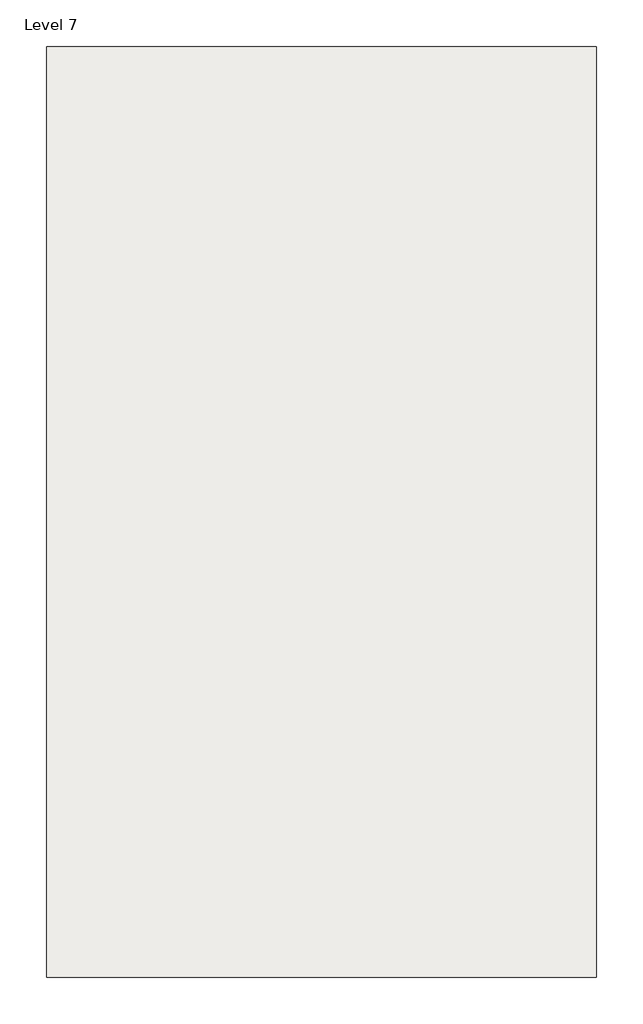
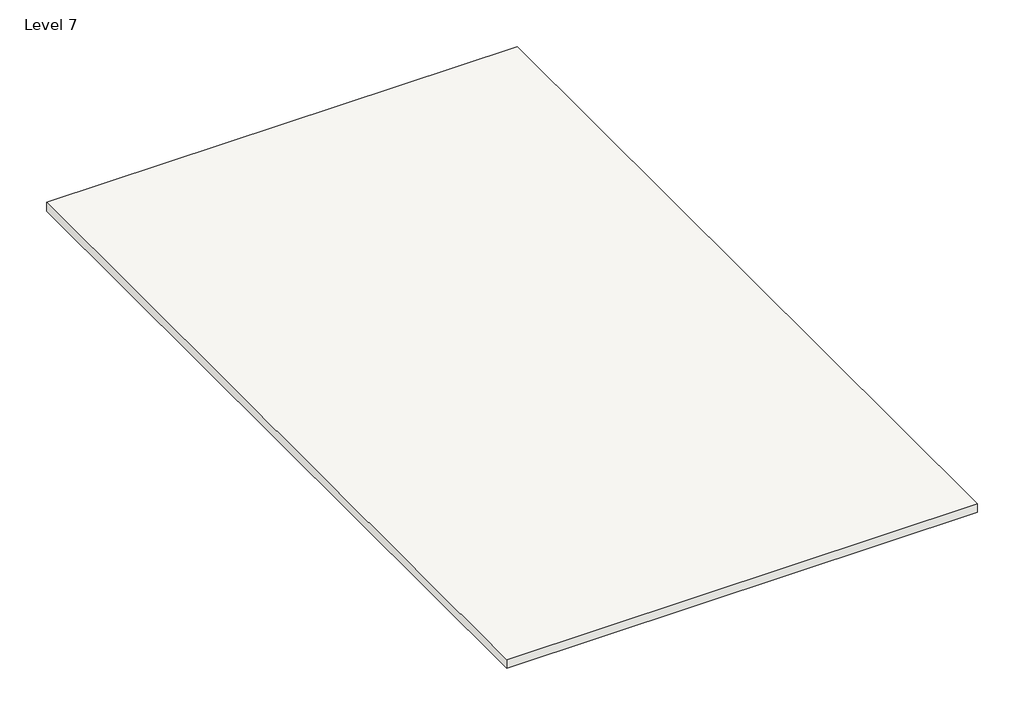
# One storey, incomplete: 1 roof.
"""IFC4 building model written with IfcOpenShell, lengths in millimetres."""

from ifc_helpers import new_model, si_unit, frame, origin, place, context, project, spatial, polyline, outline, extrude, element, save

model = new_model("IFC4")

# Units and contexts
model_context = context("Model", 3, world=origin())
ifc_project = project(units=[si_unit("LENGTHUNIT", "METRE", prefix="MILLI")], contexts=[model_context])

# Site, building, storey
site = spatial("IfcSite", under=ifc_project)
building = spatial("IfcBuilding", under=site)
storey = spatial("IfcBuildingStorey", under=building, Name="Level 7", Elevation=16002.0)

# Roof
placement = place(None, origin())
element("IfcRoof", 1, ObjectType="Generic - 12\"", at=placement, inside=storey, context=model_context, shape_type="SweptSolid", body=[
    extrude(outline(polyline([(-5222.940747, 7243.7935985), (2701.859253, 7243.7935985), (2701.859253, -6167.4064015), (-5222.940747, -6167.4064015), (-5222.940747, 7243.7935985)])), frame((0.0, 0.0, 15849.6), z_axis=(0.0, 0.0, 1.0), x_axis=(1.0, 0.0, 0.0)), (0.0, 0.0, 1.0), 152.4),
])

save(model, "model.ifc")

# Revit data of these elements
# Type "Generic - 12\""
#   Assembly Code = "B1020"
#   Layers, outside or top first: 0' - 6" no material (function 1)
# Element 1 (IfcRoof, "Generic - 12\"")
#   built-in parameter 1001705 = 52.5 (stored number, unit not read)
#   built-in parameter 1001701 = -0.5 (stored number, unit not read)
#   built-in parameter 1001710 = 33615
#   Phase Created = New Construction
#   Materials on its faces: "Default Roof", "Door - Panel"
# Materials
#   "Default Roof": colour RGB 88 101 114, transparency 0, Cost = 0
#   "Door - Panel": class "Wood", colour RGB 210 159 95, transparency 0, Cost = 0
